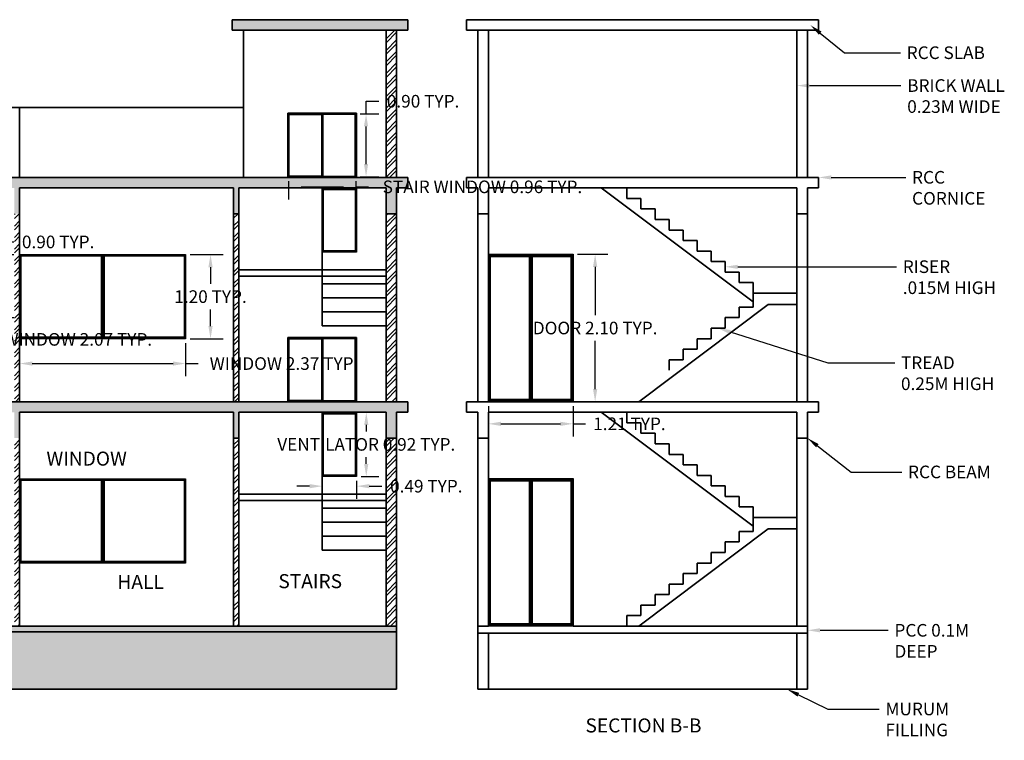
# Model space of a CAD drawing. Units: metres. Extents: x 8.1 to 56.2, y -9.3 to 36.3.
# Tile 5 of 6: x 22.5 to 36.6, y 25.7 to 36. Entities that reach past the tile are written whole.
import ezdxf
from ezdxf import colors
from ezdxf.entities.mleader import LeaderData, LeaderLine
from ezdxf.math import Vec2, Vec3

# ---------------------------------------------------------------- set-up
doc = ezdxf.new("R2010")
doc.units = ezdxf.units.M
doc.header["$LTSCALE"] = 0.01
doc.header["$MEASUREMENT"] = 0
for name, color, linetype, lineweight in [('A-ANNO-DIMS', 2, 'Continuous', 18), ('A-ANNO-TEXT', 7, 'Continuous', 18), ('A-DOOR', 4, 'Continuous', 25), ('A-GLAZ', 3, 'Continuous', 25), ('A-SECT', 7, 'Continuous', 35), ('A-SECT-PATT', 8, 'Continuous', 13)]:
    doc.layers.add(name, color=color, linetype=linetype, lineweight=lineweight)
doc.styles.get("Standard").update_dxf_attribs({"font": 'arial.ttf'})
doc.dimstyles.get("Standard").update_dxf_attribs({"dimtxt": 0.18, "dimasz": 0.18, "dimexe": 0.18, "dimexo": 0.0625, "dimgap": 0.09, "dimtad": 0, "dimtih": 1, "dimtoh": 1, "dimzin": 0, "dimdsep": 46, "dimtxsty": 'Standard', "dimcen": 0.09, "dimadec": 0, "dimazin": 0, "dimtfac": 1, "dimtofl": 0, "dimtmove": 0, "dimatfit": 3, "dimfxl": 1, "dimtolj": 1, "dimtzin": 0, "dimarcsym": 0})
pattern_1 = [(0, (-2.197816, 0), (0.023, 0.023), [0.0115, -0.0345]), (90, (-2.192066, -0.00575), (-0.023, 0.023), [0.0115, -0.0345])]
pattern_2 = [(0, (-2.197816, 0), (0.0235, 0.0235), [0.01175, -0.03525]), (90, (-2.19194, -0.005875), (-0.0235, 0.0235), [0.01175, -0.03525])]
pattern_3 = [(45, (-2.19782, 0), (-0.08220116, 0.08220116), []), (45, (-2.14301, 0), (-0.08220116, 0.08220116), [])]

# ---------------------------------------------------------------- blocks, each defined once
blk = doc.blocks.new('WIN-2400')
for p, q in [((1.164, 1.18), (1.164, 0.02)), ((1.174, 1.18), (1.174, 0.02)), ((1.184, 1.18), (1.184, 0.02)), ((1.194, 1.18), (1.194, 0.02)), ((1.204, 1.18), (1.204, 0.02))]:
    blk.add_line(p, q)
for points in [[(0, 1.2), (2.367, 1.2), (2.367, 0), (0, 0)], [(0.01, 1.19), (2.357, 1.19), (2.357, 0.01), (0.01, 0.01)], [(0.02, 1.18), (2.347, 1.18), (2.347, 0.02), (0.02, 0.02)]]:
    blk.add_lwpolyline(points, close=True)
blk = doc.blocks.new('WIN-VENT')
for points in [[(0, 0.916), (0.491, 0.916), (0.491, 0), (0, 0)], [(0.01, 0.906), (0.481, 0.906), (0.481, 0.01), (0.01, 0.01)], [(0.02, 0.896), (0.471, 0.896), (0.471, 0.02), (0.02, 0.02)]]:
    blk.add_lwpolyline(points, close=True)
blk = doc.blocks.new('DOOR-ELEV-1200')
for p, q in [((0.584, 2.074), (0.584, 0.03)), ((0.594, 2.074), (0.594, 0.03)), ((0.604, 2.074), (0.604, 0.03)), ((0.614, 2.074), (0.614, 0.03)), ((0.624, 2.074), (0.624, 0.03))]:
    blk.add_line(p, q)
for points in [[(1.208, 0), (0, 0), (0, 2.104), (1.208, 2.104)], [(1.198, 0.01), (0.01, 0.01), (0.01, 2.094), (1.198, 2.094)], [(1.188, 0.02), (0.02, 0.02), (0.02, 2.084), (1.188, 2.084)], [(1.178, 0.03), (0.03, 0.03), (0.03, 2.074), (1.178, 2.074)]]:
    blk.add_lwpolyline(points, close=True)
blk = doc.blocks.new('WIN-STAIR')
for p, q in [((0, 0), (0, 0.897)), ((0, 0.897), (0.47, 0.897)), ((0.01, 0.01), (0.01, 0.887)), ((0.01, 0.887), (0.46, 0.887)), ((0.47, 0.897), (0.47, 0.01)), ((0.961, 0.897), (0.49, 0.897)), ((0.49, 0.897), (0.49, 0.01)), ((0.951, 0.887), (0.5, 0.887)), ((0.951, 0.01), (0.951, 0.887)), ((0.961, 0), (0.961, 0.897)), ((0.47, 0), (0, 0)), ((0.46, 0.01), (0.01, 0.01)), ((0.46, 0.01), (0.951, 0.01)), ((0.47, 0), (0.961, 0))]:
    blk.add_line(p, q)
blk = doc.blocks.new('*D37')
at = {"layer": 'A-ANNO-DIMS', "color": 0, "lineweight": -2, "ltscale": 0.01, "transparency": 16777216}
for p, q in [((19.863, 31.647), (19.863, 31.219)), ((21.934, 31.647), (21.934, 31.219)), ((20.043, 31.399), (21.754, 31.399)), ((21.934, 31.399), (22.114, 31.399))]:
    blk.add_line(p, q, dxfattribs=at)
at = {"layer": 'A-ANNO-DIMS', "color": 0, "ltscale": 0.01, "transparency": 16777216}
for points in [[(20.043, 31.429), (20.043, 31.369), (19.863, 31.399)], [(21.754, 31.429), (21.754, 31.369), (21.934, 31.399)]]:
    blk.add_solid(points, dxfattribs=at)
at = {"layer": 'Defpoints', "color": 0, "ltscale": 0.01, "transparency": 16777216}
for p in [(19.863, 31.709), (21.934, 31.709), (21.934, 31.399)]:
    blk.add_point(p, dxfattribs=at)
at = {"layer": 'A-ANNO-DIMS', "color": 0, "ltscale": 0.01, "transparency": 16777216, "insert": (23.337, 31.399), "char_height": 0.18, "attachment_point": 5}
blk.add_mtext('\\A1;WINDOW 2.07 TYP.', dxfattribs=at)
blk = doc.blocks.new('*D38')
at = {"layer": 'A-ANNO-DIMS', "color": 0, "lineweight": -2, "ltscale": 0.01, "transparency": 16777216}
for p, q in [((22.244, 32.609), (22.244, 32.789)), ((22.244, 32.789), (22.424, 32.789)), ((21.996, 32.609), (22.424, 32.609)), ((22.244, 31.889), (22.244, 32.429)), ((21.996, 31.709), (22.424, 31.709))]:
    blk.add_line(p, q, dxfattribs=at)
at = {"layer": 'A-ANNO-DIMS', "color": 0, "ltscale": 0.01, "transparency": 16777216}
for points in [[(22.214, 32.429), (22.274, 32.429), (22.244, 32.609)], [(22.214, 31.889), (22.274, 31.889), (22.244, 31.709)]]:
    blk.add_solid(points, dxfattribs=at)
at = {"layer": 'Defpoints', "color": 0, "ltscale": 0.01, "transparency": 16777216}
for p in [(21.934, 32.609), (22.244, 32.609), (21.934, 31.709)]:
    blk.add_point(p, dxfattribs=at)
at = {"layer": 'A-ANNO-DIMS', "color": 0, "ltscale": 0.01, "transparency": 16777216, "insert": (23.057, 32.789), "char_height": 0.18, "attachment_point": 5}
blk.add_mtext('\\A1;0.90 TYP.', dxfattribs=at)
blk = doc.blocks.new('*D39')
at = {"layer": 'A-ANNO-DIMS', "color": 0, "lineweight": -2, "ltscale": 0.01, "transparency": 16777216}
for p, q in [((22.508, 31.347), (22.508, 30.874)), ((24.875, 31.347), (24.875, 30.874)), ((22.688, 31.054), (24.695, 31.054)), ((24.875, 31.054), (25.055, 31.054))]:
    blk.add_line(p, q, dxfattribs=at)
at = {"layer": 'A-ANNO-DIMS', "color": 0, "ltscale": 0.01, "transparency": 16777216}
for points in [[(22.688, 31.084), (22.688, 31.024), (22.508, 31.054)], [(24.695, 31.084), (24.695, 31.024), (24.875, 31.054)]]:
    blk.add_solid(points, dxfattribs=at)
at = {"layer": 'Defpoints', "color": 0, "ltscale": 0.01, "transparency": 16777216}
for p in [(22.508, 31.409), (24.875, 31.409), (24.875, 31.054)]:
    blk.add_point(p, dxfattribs=at)
at = {"layer": 'A-ANNO-DIMS', "color": 0, "ltscale": 0.01, "transparency": 16777216, "insert": (26.278, 31.054), "char_height": 0.18, "attachment_point": 5}
blk.add_mtext('\\A1;WINDOW 2.37 TYP.', dxfattribs=at)
blk = doc.blocks.new('*D40')
at = {"layer": 'A-ANNO-DIMS', "color": 0, "lineweight": -2, "ltscale": 0.01, "transparency": 16777216}
for p, q in [((24.938, 32.609), (25.41, 32.609)), ((25.23, 32.429), (25.23, 32.191)), ((25.23, 31.589), (25.23, 31.827)), ((24.938, 31.409), (25.41, 31.409))]:
    blk.add_line(p, q, dxfattribs=at)
at = {"layer": 'A-ANNO-DIMS', "color": 0, "ltscale": 0.01, "transparency": 16777216}
for points in [[(25.2, 32.429), (25.26, 32.429), (25.23, 32.609)], [(25.2, 31.589), (25.26, 31.589), (25.23, 31.409)]]:
    blk.add_solid(points, dxfattribs=at)
at = {"layer": 'Defpoints', "color": 0, "ltscale": 0.01, "transparency": 16777216}
for p in [(24.875, 32.609), (25.23, 32.609), (24.875, 31.409)]:
    blk.add_point(p, dxfattribs=at)
at = {"layer": 'A-ANNO-DIMS', "color": 0, "ltscale": 0.01, "transparency": 16777216, "insert": (25.23, 32.009), "char_height": 0.18, "attachment_point": 5}
blk.add_mtext('\\A1;1.20 TYP.', dxfattribs=at)
blk = doc.blocks.new('*D41')
at = {"layer": 'A-ANNO-DIMS', "color": 0, "lineweight": -2, "ltscale": 0.01, "transparency": 16777216}
for p, q in [((27.376, 30.359), (27.631, 30.359)), ((27.451, 30.179), (27.451, 30.084)), ((27.451, 29.623), (27.451, 29.718)), ((27.376, 29.443), (27.631, 29.443))]:
    blk.add_line(p, q, dxfattribs=at)
at = {"layer": 'A-ANNO-DIMS', "color": 0, "ltscale": 0.01, "transparency": 16777216}
for points in [[(27.421, 30.179), (27.481, 30.179), (27.451, 30.359)], [(27.421, 29.623), (27.481, 29.623), (27.451, 29.443)]]:
    blk.add_solid(points, dxfattribs=at)
at = {"layer": 'Defpoints', "color": 0, "ltscale": 0.01, "transparency": 16777216}
for p in [(27.314, 30.359), (27.451, 30.359), (27.314, 29.443)]:
    blk.add_point(p, dxfattribs=at)
at = {"layer": 'A-ANNO-DIMS', "color": 0, "ltscale": 0.01, "transparency": 16777216, "insert": (27.451, 29.901), "char_height": 0.18, "attachment_point": 5}
blk.add_mtext('\\A1;VENTILATOR 0.92 TYP.', dxfattribs=at)
blk = doc.blocks.new('*D42')
at = {"layer": 'A-ANNO-DIMS', "color": 0, "lineweight": -2, "ltscale": 0.01, "transparency": 16777216}
for p, q in [((26.823, 29.38), (26.823, 29.125)), ((27.314, 29.38), (27.314, 29.125)), ((26.643, 29.305), (26.463, 29.305)), ((27.494, 29.305), (27.674, 29.305))]:
    blk.add_line(p, q, dxfattribs=at)
at = {"layer": 'A-ANNO-DIMS', "color": 0, "ltscale": 0.01, "transparency": 16777216}
for points in [[(26.643, 29.335), (26.643, 29.275), (26.823, 29.305)], [(27.494, 29.335), (27.494, 29.275), (27.314, 29.305)]]:
    blk.add_solid(points, dxfattribs=at)
at = {"layer": 'Defpoints', "color": 0, "ltscale": 0.01, "transparency": 16777216}
for p in [(26.823, 29.443), (27.314, 29.443), (27.314, 29.305)]:
    blk.add_point(p, dxfattribs=at)
at = {"layer": 'A-ANNO-DIMS', "color": 0, "ltscale": 0.01, "transparency": 16777216, "insert": (28.307, 29.305), "char_height": 0.18, "attachment_point": 5}
blk.add_mtext('\\A1;0.49 TYP.', dxfattribs=at)
blk = doc.blocks.new('*D43')
at = {"layer": 'A-ANNO-DIMS', "color": 0, "lineweight": -2, "ltscale": 0.01, "transparency": 16777216}
for p, q in [((26.343, 33.657), (26.343, 33.395)), ((26.523, 33.575), (27.124, 33.575)), ((27.304, 33.657), (27.304, 33.395)), ((27.304, 33.575), (27.484, 33.575))]:
    blk.add_line(p, q, dxfattribs=at)
at = {"layer": 'A-ANNO-DIMS', "color": 0, "ltscale": 0.01, "transparency": 16777216}
for points in [[(26.523, 33.605), (26.523, 33.545), (26.343, 33.575)], [(27.124, 33.605), (27.124, 33.545), (27.304, 33.575)]]:
    blk.add_solid(points, dxfattribs=at)
at = {"layer": 'Defpoints', "color": 0, "ltscale": 0.01, "transparency": 16777216}
for p in [(26.343, 33.719), (27.304, 33.719), (27.304, 33.575)]:
    blk.add_point(p, dxfattribs=at)
at = {"layer": 'A-ANNO-DIMS', "color": 0, "ltscale": 0.01, "transparency": 16777216, "insert": (29.108, 33.575), "char_height": 0.18, "attachment_point": 5}
blk.add_mtext('\\A1;STAIR WINDOW 0.96 TYP.', dxfattribs=at)
blk = doc.blocks.new('*D44')
at = {"layer": 'A-ANNO-DIMS', "color": 0, "lineweight": -2, "ltscale": 0.01, "transparency": 16777216}
for p, q in [((27.448, 34.616), (27.448, 34.796)), ((27.448, 34.796), (27.628, 34.796)), ((27.366, 34.616), (27.628, 34.616)), ((27.448, 33.899), (27.448, 34.436)), ((27.366, 33.719), (27.628, 33.719))]:
    blk.add_line(p, q, dxfattribs=at)
at = {"layer": 'A-ANNO-DIMS', "color": 0, "ltscale": 0.01, "transparency": 16777216}
for points in [[(27.418, 34.436), (27.478, 34.436), (27.448, 34.616)], [(27.418, 33.899), (27.478, 33.899), (27.448, 33.719)]]:
    blk.add_solid(points, dxfattribs=at)
at = {"layer": 'Defpoints', "color": 0, "ltscale": 0.01, "transparency": 16777216}
for p in [(27.304, 34.616), (27.448, 34.616), (27.304, 33.719)]:
    blk.add_point(p, dxfattribs=at)
at = {"layer": 'A-ANNO-DIMS', "color": 0, "ltscale": 0.01, "transparency": 16777216, "insert": (28.261, 34.796), "char_height": 0.18, "attachment_point": 5}
blk.add_mtext('\\A1;0.90 TYP.', dxfattribs=at)
blk = doc.blocks.new('*D45')
at = {"layer": 'A-ANNO-DIMS', "color": 0, "lineweight": -2, "ltscale": 0.01, "transparency": 16777216}
for p, q in [((30.462, 32.613), (30.895, 32.613)), ((30.715, 32.433), (30.715, 31.744)), ((30.715, 30.689), (30.715, 31.378)), ((30.462, 30.509), (30.895, 30.509))]:
    blk.add_line(p, q, dxfattribs=at)
at = {"layer": 'A-ANNO-DIMS', "color": 0, "ltscale": 0.01, "transparency": 16777216}
for points in [[(30.685, 32.433), (30.745, 32.433), (30.715, 32.613)], [(30.685, 30.689), (30.745, 30.689), (30.715, 30.509)]]:
    blk.add_solid(points, dxfattribs=at)
at = {"layer": 'Defpoints', "color": 0, "ltscale": 0.01, "transparency": 16777216}
for p in [(30.4, 32.613), (30.715, 32.613), (30.4, 30.509)]:
    blk.add_point(p, dxfattribs=at)
at = {"layer": 'A-ANNO-DIMS', "color": 0, "ltscale": 0.01, "transparency": 16777216, "insert": (30.715, 31.561), "char_height": 0.18, "attachment_point": 5}
blk.add_mtext('\\A1;DOOR 2.10 TYP.', dxfattribs=at)
blk = doc.blocks.new('*D46')
at = {"layer": 'A-ANNO-DIMS', "color": 0, "lineweight": -2, "ltscale": 0.01, "transparency": 16777216}
for p, q in [((29.192, 30.447), (29.192, 30.014)), ((30.4, 30.447), (30.4, 30.014)), ((29.372, 30.194), (30.22, 30.194)), ((30.4, 30.194), (30.58, 30.194))]:
    blk.add_line(p, q, dxfattribs=at)
at = {"layer": 'A-ANNO-DIMS', "color": 0, "ltscale": 0.01, "transparency": 16777216}
for points in [[(29.372, 30.224), (29.372, 30.164), (29.192, 30.194)], [(30.22, 30.224), (30.22, 30.164), (30.4, 30.194)]]:
    blk.add_solid(points, dxfattribs=at)
at = {"layer": 'Defpoints', "color": 0, "ltscale": 0.01, "transparency": 16777216}
for p in [(29.192, 30.509), (30.4, 30.509), (30.4, 30.194)]:
    blk.add_point(p, dxfattribs=at)
at = {"layer": 'A-ANNO-DIMS', "color": 0, "ltscale": 0.01, "transparency": 16777216, "insert": (31.204, 30.194), "char_height": 0.18, "attachment_point": 5}
blk.add_mtext('\\A1;1.21 TYP.', dxfattribs=at)

msp = doc.modelspace()

# ---------------------------------------------------------------- hatches: boundary and pattern name
at = {"layer": 'A-SECT-PATT'}
h = msp.add_hatch(dxfattribs=at)
h.set_pattern_fill('CROSS', color=256, scale=0.094)
h.set_pattern_definition(pattern_2)
h.paths.add_polyline_path([(25.701, 35.959), (25.54, 35.959), (25.54, 35.809), (25.701, 35.809), (27.883, 35.809), (28.044, 35.809), (28.044, 35.959), (27.883, 35.959)])
h = msp.add_hatch(dxfattribs=at)
h.set_pattern_fill('ANSI32', color=256, scale=0.31)
h.set_pattern_definition(pattern_3)
h.paths.add_polyline_path([(27.733, 33.709), (27.883, 33.709), (27.883, 35.809), (27.733, 35.809)])
h = msp.add_hatch(dxfattribs=at)
h.set_pattern_fill('CROSS', color=256, scale=0.094)
h.set_pattern_definition(pattern_2)
h.paths.add_polyline_path([(15.663, 33.709), (15.503, 33.709), (15.503, 33.559), (15.663, 33.559), (15.663, 33.192), (15.813, 33.192), (15.813, 33.559), (17.013, 33.559), (17.013, 33.192), (17.088, 33.192), (17.088, 33.559), (19.788, 33.559), (19.788, 33.192), (19.863, 33.192), (19.863, 33.559), (22.433, 33.559), (22.433, 33.192), (22.508, 33.192), (22.508, 33.559), (25.558, 33.559), (25.558, 33.192), (25.633, 33.192), (25.633, 33.559), (27.733, 33.559), (27.733, 33.192), (27.883, 33.192), (27.883, 33.559), (28.044, 33.559), (28.044, 33.709), (27.883, 33.709)])
h = msp.add_hatch(dxfattribs=at)
h.set_pattern_fill('ANSI32', color=256, scale=0.31)
h.set_pattern_definition(pattern_3)
h.paths.add_polyline_path([(19.863, 33.192), (19.788, 33.192), (19.788, 30.509), (19.863, 30.509)])
h.paths.add_polyline_path([(22.508, 33.192), (22.433, 33.192), (22.433, 30.509), (22.508, 30.509)])
h.paths.add_polyline_path([(25.633, 33.192), (25.558, 33.192), (25.558, 30.509), (25.633, 30.509)])
h.paths.add_polyline_path([(27.883, 33.192), (27.733, 33.192), (27.733, 30.509), (27.883, 30.509)])
h.paths.add_polyline_path([(27.733, 27.309), (27.883, 27.309), (27.883, 29.992), (27.733, 29.992)])
h.paths.add_polyline_path([(25.558, 27.309), (25.633, 27.309), (25.633, 29.992), (25.558, 29.992)])
h = msp.add_hatch(dxfattribs=at)
h.set_pattern_fill('CROSS', color=256, scale=0.092)
h.set_pattern_definition(pattern_1)
h.paths.add_polyline_path([(17.013, 30.359), (17.013, 29.992), (17.088, 29.992), (17.088, 30.359), (19.788, 30.359), (19.788, 29.992), (19.863, 29.992), (19.863, 30.359), (22.433, 30.359), (22.433, 29.992), (22.508, 29.992), (22.508, 30.359), (25.558, 30.359), (25.558, 29.992), (25.633, 29.992), (25.633, 30.359), (27.733, 30.359), (27.733, 29.992), (27.883, 29.992), (27.883, 30.359), (28.044, 30.359), (28.044, 30.509), (27.883, 30.509), (15.663, 30.509), (15.503, 30.509), (15.503, 30.359), (15.663, 30.359), (15.663, 29.992), (15.813, 29.992), (15.813, 30.359)])
h = msp.add_hatch(dxfattribs=at)
h.set_pattern_fill('ANSI32', color=256, scale=0.31)
h.set_pattern_definition(pattern_3)
h.paths.add_polyline_path([(22.433, 27.309), (22.508, 27.309), (22.508, 29.992), (22.433, 29.992)])
h.paths.add_polyline_path([(19.788, 27.309), (19.863, 27.309), (19.863, 29.992), (19.788, 29.992)])
h.paths.add_polyline_path([(17.013, 27.309), (17.088, 27.309), (17.088, 29.992), (17.013, 29.992)])
h.paths.add_polyline_path([(15.663, 27.309), (15.813, 27.309), (15.813, 29.992), (15.663, 29.992)])
h = msp.add_hatch(dxfattribs=at)
h.set_pattern_fill('CROSS', color=256, scale=0.092)
h.set_pattern_definition(pattern_1)
h.paths.add_polyline_path([(15.663, 27.309), (15.663, 27.229), (27.883, 27.229), (27.883, 27.309)])
h = msp.add_hatch(dxfattribs=at)
h.set_pattern_fill('GRAVEL', color=256, scale=0.7)
h.set_pattern_definition([(228.01279, (-1.693816, 0.7), (-5.6, -6.3), [0.094175, -9.323362]), (184.96974, (-1.756816, 0.63), (8.4, 0.7), [0.161608, -15.999147]), (132.51045, (-1.917816, 0.616), (7, -7.7), [0.113952, -11.281223]), (267.27369, (-2.190816, 0.441), (0.7, 14), [0.147167, -14.569491]), (292.83365, (-2.197816, 0.294), (-3.5, 8.4), [0.1443085, -14.286561]), (357.27369, (-2.141816, 0.161), (-14, 0.7), [0.147167, -14.569491]), (37.69424, (-1.994816, 0.154), (-9.1, -7), [0.19462, -19.267394]), (72.25533, (-1.840816, 0.273), (4.9, 15.4), [0.183742, -18.190425]), (121.42957, (-1.784816, 0.448), (-5.6, 9.1), [0.147665, -14.618851]), (175.23636, (-1.861816, 0.574), (7.7, -0.7), [0.168582, -8.260534]), (222.39744, (-2.029816, 0.588), (-8.4, -7.7), [0.2180136, -21.5833625]), (138.81407, (-1.497816, 0.434), (-4.9, 4.2), [0.074411, -7.366691]), (171.46923, (-1.553816, 0.483), (9.1, -1.4), [0.141566, -14.015058]), (225, (-1.6938, 0.504), (-1e-16, -0.7), [0.098995, -0.890955]), (203.1986, (-1.74282, 0.588), (3.5, 1.4), [0.053311, -5.277731]), (291.8014, (-1.79182, 0.567), (-0.7, 2.1), [0.075392, -3.694223]), (30.96376, (-1.76382, 0.497), (2.1, 1.4), [0.12245, -3.959216]), (161.56505, (-1.65882, 0.56), (1.4, -0.7), [0.088544, -2.125051]), (16.38954, (-2.197816, 0.567), (7, 2.1), [0.12404, -12.279992]), (70.34618, (-2.078816, 0.602), (-2.8, -7.7), [0.104063, -10.302185]), (293.1986, (-1.65882, 0.7), (-1.4, 3.5), [0.10662, -5.224421]), (343.61046, (-1.616816, 0.602), (-7, 2.1), [0.12404, -12.279992]), (339.44395, (-2.197816, 0.133), (-3.5, 1.4), [0.119616, -5.861187]), (294.77514, (-2.085816, 0.091), (-3.5, 7.7), [0.100225, -9.92225]), (66.8014, (-1.65182, 0), (1.4, 3.5), [0.10662, -5.224421]), (17.35402, (-1.609816, 0.098), (-9.1, -2.8), [0.117342, -11.616797]), (69.44395, (-1.994816, 0), (-1.4, -3.5), [0.059808, -5.920995]), (101.30993, (-1.69382, 0), (-0.7, 2.8), [0.035693, -3.533621]), (165.96376, (-1.70082, 0.035), (2.1, -0.7), [0.144309, -2.741865]), (186.00901, (-1.840816, 0.07), (7, 0.7), [0.133735, -13.239746]), (303.69007, (-1.76382, 0.434), (-0.7, 1.4), [0.100955, -2.42293]), (353.15723, (-1.707816, 0.35), (11.9, -1.4), [0.176256, -17.449294]), (60.9454, (-1.532816, 0.329), (-2.8, -4.9), [0.072069, -7.134872]), (90, (-1.4978, 0.392), (-0.7, 0.7), [0.042, -0.658]), (120.25644, (-1.854816, 0.091), (2.8, -4.9), [0.097247, -9.627464]), (48.01279, (-1.903816, 0.175), (5.6, 6.3), [0.18835, -9.229186]), (0, (-1.7778, 0.315), (0.7, 0.7), [0.182, -0.518]), (325.30485, (-1.595816, 0.315), (7, -4.9), [0.11068, -10.957292]), (254.0546, (-1.50482, 0.252), (-0.7, -2.8), [0.101921, -4.994156]), (207.645975, (-1.532816, 0.154), (-13.3, -7), [0.1659455, -16.428632]), (175.42608, (-1.679816, 0.077), (-9.1, 0.7), [0.175559, -17.380351])])
h.paths.add_polyline_path([(27.883, 26.409), (27.883, 27.229), (15.663, 27.229), (15.663, 26.409)])

# ---------------------------------------------------------------- linework, layer by layer
at = {"layer": 'A-SECT'}
for p, q in [((25.701, 35.959), (25.54, 35.959)), ((25.54, 35.959), (25.54, 35.809)), ((27.883, 35.959), (25.701, 35.959)), ((27.883, 35.959), (28.044, 35.959)), ((28.044, 35.959), (28.044, 35.809)), ((29.042, 35.959), (28.881, 35.959)), ((28.881, 35.959), (28.881, 35.809)), ((33.742, 35.959), (29.042, 35.959)), ((33.742, 35.959), (33.902, 35.959)), ((33.902, 35.959), (33.902, 35.809)), ((25.54, 35.809), (25.701, 35.809)), ((25.701, 35.809), (25.701, 33.709)), ((27.883, 35.809), (25.701, 35.809)), ((27.733, 33.709), (27.733, 35.809)), ((27.883, 33.709), (27.883, 35.809)), ((28.044, 35.809), (27.883, 35.809)), ((28.881, 35.809), (29.042, 35.809)), ((29.042, 35.809), (29.042, 33.709)), ((33.742, 35.809), (29.042, 35.809)), ((29.192, 35.809), (29.192, 33.709)), ((33.592, 33.709), (33.592, 35.809)), ((33.742, 33.709), (33.742, 35.809)), ((33.902, 35.809), (33.742, 35.809)), ((15.663, 34.709), (25.701, 34.709)), ((22.508, 33.709), (22.508, 34.709)), ((26.333, 33.709), (26.333, 34.626)), ((26.333, 34.626), (26.823, 34.626)), ((27.314, 34.626), (26.823, 34.626)), ((26.823, 34.626), (26.823, 33.729)), ((26.823, 34.626), (26.823, 33.729)), ((27.314, 33.709), (27.314, 34.626)), ((15.663, 33.709), (27.883, 33.709)), ((27.883, 33.709), (28.044, 33.709)), ((28.044, 33.709), (28.044, 33.559)), ((29.042, 33.709), (28.881, 33.709)), ((28.881, 33.709), (28.881, 33.559)), ((29.042, 33.709), (33.742, 33.709)), ((33.742, 33.709), (33.902, 33.709)), ((33.902, 33.709), (33.902, 33.559)), ((22.508, 30.509), (22.508, 33.559)), ((22.508, 33.559), (25.558, 33.559)), ((25.558, 30.509), (25.558, 33.559)), ((25.633, 30.509), (25.633, 33.559)), ((25.633, 33.559), (27.733, 33.559)), ((26.823, 32.393), (26.823, 33.559)), ((27.733, 30.509), (27.733, 33.559)), ((27.883, 30.509), (27.883, 33.559)), ((28.044, 33.559), (27.883, 33.559)), ((28.881, 33.559), (29.042, 33.559)), ((29.042, 30.509), (29.042, 33.559)), ((29.192, 30.509), (29.192, 33.559)), ((29.192, 33.559), (33.592, 33.559)), ((31.169, 33.559), (31.169, 33.409)), ((33.592, 30.509), (33.592, 33.559)), ((33.742, 30.509), (33.742, 33.559)), ((33.902, 33.559), (33.742, 33.559)), ((31.169, 33.409), (31.369, 33.409)), ((31.369, 33.409), (31.369, 33.259)), ((25.558, 33.192), (25.633, 33.192)), ((27.733, 33.192), (27.883, 33.192)), ((29.042, 33.192), (29.192, 33.192)), ((31.369, 33.259), (31.569, 33.259)), ((31.569, 33.259), (31.569, 33.109)), ((33.592, 33.192), (33.742, 33.192)), ((31.569, 33.109), (31.769, 33.109)), ((31.769, 33.109), (31.769, 32.959)), ((31.769, 32.959), (31.969, 32.959)), ((31.969, 32.959), (31.969, 32.809)), ((31.969, 32.809), (32.169, 32.809)), ((32.169, 32.809), (32.169, 32.659)), ((32.169, 32.659), (32.369, 32.659)), ((32.369, 32.659), (32.369, 32.509)), ((32.369, 32.509), (32.569, 32.509)), ((32.569, 32.509), (32.569, 32.359)), ((26.823, 32.393), (25.633, 32.393)), ((27.733, 32.3), (25.633, 32.3)), ((27.733, 32.393), (26.823, 32.393)), ((26.823, 31.593), (26.823, 32.393)), ((32.569, 32.359), (32.769, 32.359)), ((32.769, 32.359), (32.769, 32.209)), ((27.733, 32.193), (26.823, 32.193)), ((32.769, 32.209), (32.969, 32.209)), ((32.969, 32.209), (32.969, 32.059)), ((32.969, 32.059), (33.592, 32.059)), ((32.969, 32.059), (32.969, 32.009)), ((27.733, 31.993), (26.823, 31.993)), ((32.969, 32.009), (32.969, 31.859)), ((33.184, 31.896), (33.592, 31.896)), ((27.733, 31.793), (26.823, 31.793)), ((32.969, 31.859), (32.769, 31.859)), ((32.769, 31.859), (32.769, 31.709)), ((32.769, 31.709), (32.569, 31.709)), ((32.569, 31.709), (32.569, 31.559)), ((27.733, 31.593), (26.823, 31.593)), ((32.569, 31.559), (32.369, 31.559)), ((32.369, 31.559), (32.369, 31.409)), ((26.333, 30.509), (26.333, 31.426)), ((26.333, 31.426), (26.823, 31.426)), ((27.314, 31.426), (26.823, 31.426)), ((26.823, 31.426), (26.823, 30.529)), ((26.823, 31.426), (26.823, 30.529)), ((27.314, 30.509), (27.314, 31.426)), ((32.369, 31.409), (32.169, 31.409)), ((32.169, 31.409), (32.169, 31.259)), ((32.169, 31.259), (31.969, 31.259)), ((31.969, 31.259), (31.969, 31.109)), ((31.969, 31.109), (31.769, 31.109)), ((31.769, 31.109), (31.769, 30.959)), ((15.663, 30.509), (27.883, 30.509)), ((26.823, 30.509), (26.333, 30.509)), ((26.823, 30.509), (27.314, 30.509)), ((27.883, 30.509), (28.044, 30.509)), ((28.044, 30.509), (28.044, 30.359)), ((29.042, 30.509), (28.881, 30.509)), ((28.881, 30.509), (28.881, 30.359)), ((29.042, 30.509), (33.742, 30.509)), ((33.742, 30.509), (33.902, 30.509)), ((33.902, 30.509), (33.902, 30.359)), ((22.508, 27.309), (22.508, 30.359)), ((22.508, 30.359), (25.558, 30.359)), ((25.558, 27.309), (25.558, 30.359)), ((25.633, 27.309), (25.633, 30.359)), ((25.633, 30.359), (27.733, 30.359)), ((26.823, 29.193), (26.823, 30.359)), ((27.733, 27.309), (27.733, 30.359)), ((27.883, 27.309), (27.883, 30.359)), ((28.044, 30.359), (27.883, 30.359)), ((28.881, 30.359), (29.042, 30.359)), ((29.042, 27.309), (29.042, 30.359)), ((29.192, 27.309), (29.192, 30.359)), ((29.192, 30.359), (33.592, 30.359)), ((31.169, 30.359), (31.169, 30.209)), ((33.592, 27.309), (33.592, 30.359)), ((33.742, 27.309), (33.742, 30.359)), ((33.902, 30.359), (33.742, 30.359)), ((31.169, 30.209), (31.369, 30.209)), ((31.369, 30.209), (31.369, 30.059)), ((31.369, 30.059), (31.569, 30.059)), ((31.569, 30.059), (31.569, 29.909)), ((25.558, 29.992), (25.633, 29.992)), ((27.733, 29.992), (27.883, 29.992)), ((29.042, 29.992), (29.192, 29.992)), ((33.592, 29.992), (33.742, 29.992)), ((31.569, 29.909), (31.769, 29.909)), ((31.769, 29.909), (31.769, 29.759)), ((31.769, 29.759), (31.969, 29.759)), ((31.969, 29.759), (31.969, 29.609)), ((31.969, 29.609), (32.169, 29.609)), ((32.169, 29.609), (32.169, 29.459)), ((32.169, 29.459), (32.369, 29.459)), ((32.369, 29.459), (32.369, 29.309)), ((32.369, 29.309), (32.569, 29.309)), ((32.569, 29.309), (32.569, 29.159)), ((26.823, 29.193), (25.633, 29.193)), ((27.733, 29.1), (25.633, 29.1)), ((27.733, 29.193), (26.823, 29.193)), ((26.823, 28.393), (26.823, 29.193)), ((32.569, 29.159), (32.769, 29.159)), ((32.769, 29.159), (32.769, 29.009)), ((27.733, 28.993), (26.823, 28.993)), ((32.769, 29.009), (32.969, 29.009)), ((32.969, 29.009), (32.969, 28.859)), ((27.733, 28.793), (26.823, 28.793)), ((32.969, 28.859), (33.592, 28.859)), ((32.969, 28.859), (32.969, 28.809)), ((32.969, 28.809), (32.969, 28.659)), ((32.969, 28.659), (32.769, 28.659)), ((32.769, 28.659), (32.769, 28.509)), ((33.184, 28.696), (33.592, 28.696)), ((27.733, 28.593), (26.823, 28.593)), ((32.769, 28.509), (32.569, 28.509)), ((32.569, 28.509), (32.569, 28.359)), ((27.733, 28.393), (26.823, 28.393)), ((32.569, 28.359), (32.369, 28.359)), ((32.369, 28.359), (32.369, 28.209)), ((32.369, 28.209), (32.169, 28.209)), ((32.169, 28.209), (32.169, 28.059)), ((32.169, 28.059), (31.969, 28.059)), ((31.969, 28.059), (31.969, 27.909)), ((31.969, 27.909), (31.769, 27.909)), ((31.769, 27.909), (31.769, 27.759)), ((31.769, 27.759), (31.569, 27.759)), ((31.569, 27.759), (31.569, 27.609)), ((31.569, 27.609), (31.369, 27.609)), ((31.369, 27.609), (31.369, 27.459)), ((31.369, 27.459), (31.169, 27.459)), ((31.169, 27.459), (31.169, 27.309)), ((15.663, 27.309), (27.883, 27.309)), ((27.883, 27.309), (27.883, 26.409)), ((29.042, 26.409), (29.042, 27.309)), ((29.192, 27.309), (29.042, 27.309)), ((30.4, 27.309), (33.742, 27.309)), ((33.742, 27.309), (33.742, 26.409)), ((15.663, 27.229), (27.883, 27.229)), ((29.042, 27.209), (33.742, 27.209)), ((29.192, 26.409), (29.192, 27.209)), ((33.592, 27.209), (33.592, 26.409)), ((15.663, 26.409), (27.883, 26.409)), ((29.042, 26.409), (33.742, 26.409))]:
    msp.add_line(p, q, dxfattribs=at)
for points in [[(30.802, 33.559), (32.969, 31.934)], [(33.184, 31.896), (31.336, 30.509)], [(30.802, 30.359), (32.969, 28.734)], [(33.184, 28.696), (31.336, 27.309)]]:
    msp.add_lwpolyline(points, dxfattribs=at)

# ---------------------------------------------------------------- block references
at = {"layer": 'A-DOOR'}
for p in [(29.192, 30.509), (29.192, 27.309)]:
    msp.add_blockref('DOOR-ELEV-1200', p, dxfattribs=at)
at = {"layer": 'A-GLAZ'}
for name, p in [('WIN-STAIR', (26.343, 33.719)), ('WIN-VENT', (26.823, 32.643)), ('WIN-2400', (22.508, 31.409)), ('WIN-STAIR', (26.343, 30.519)), ('WIN-VENT', (26.823, 29.443)), ('WIN-2400', (22.508, 28.209))]:
    msp.add_blockref(name, p, dxfattribs=at)

# ---------------------------------------------------------------- texts
at = {"layer": 'A-ANNO-TEXT', "char_height": 0.2, "attachment_point": 1}
for s, width, insert in [('WINDOW', 1.61769, (22.89, 29.798)), ('\\pxqc;HALL', 1.61769, (23.424, 28.04)), ('\\pxqc;STAIRS', 1.61769, (25.843, 28.05)), ('\\pxqc;SECTION B-B', 4.05553, (29.377, 25.992))]:
    msp.add_mtext_dynamic_manual_height_columns(s, width=width, gutter_width=1, heights=[0], dxfattribs=dict(at, insert=insert))

# ---------------------------------------------------------------- dimensions: what is measured, and where the dimension line sits
at = {"layer": 'A-ANNO-DIMS', "ltscale": 0.01}
for base, p1, p2, text, picture, middle in [((27.448, 34.616), (27.304, 33.719), (27.304, 34.616), '<> TYP.', '*D44', (28.261, 34.796)), ((22.244, 32.609), (21.934, 31.709), (21.934, 32.609), '<> TYP.', '*D38', (23.057, 32.789)), ((25.23, 32.609), (24.875, 31.409), (24.875, 32.609), '<> TYP.', '*D40', (25.23, 32.009)), ((30.715, 32.613), (30.4, 30.509), (30.4, 32.613), 'DOOR <> TYP.', '*D45', (30.715, 31.561)), ((27.451, 30.359), (27.314, 29.443), (27.314, 30.359), 'VENTILATOR <> TYP.', '*D41', (27.451, 29.901))]:
    dim = msp.add_linear_dim(base=base, p1=p1, p2=p2, angle=90, text=text, dimstyle='Standard', override={"dimdec": 2, "dimrnd": 0, "dimzin": 0, "dimlunit": 2}, dxfattribs=at)
    dim.commit()
    dim.dimension.update_dxf_attribs({"geometry": picture, "text_midpoint": middle})
for base, p1, p2, text, picture, middle in [((27.304, 33.575), (26.343, 33.719), (27.304, 33.719), 'STAIR WINDOW <> TYP.', '*D43', (29.108, 33.575)), ((21.934, 31.399), (19.863, 31.709), (21.934, 31.709), 'WINDOW <> TYP.', '*D37', (23.337, 31.399)), ((24.875, 31.054), (22.508, 31.409), (24.875, 31.409), 'WINDOW <> TYP.', '*D39', (26.278, 31.054)), ((30.4, 30.194), (29.192, 30.509), (30.4, 30.509), '<> TYP.', '*D46', (31.204, 30.194)), ((27.314, 29.305), (26.823, 29.443), (27.314, 29.443), '<> TYP.', '*D42', (28.307, 29.305))]:
    dim = msp.add_linear_dim(base=base, p1=p1, p2=p2, text=text, dimstyle='Standard', override={"dimdec": 2, "dimrnd": 0, "dimzin": 0, "dimlunit": 2}, dxfattribs=at)
    dim.commit()
    dim.dimension.update_dxf_attribs({"geometry": picture, "text_midpoint": middle})

# ---------------------------------------------------------------- leaders
at = {"layer": 'A-ANNO-TEXT'}
ml = msp.add_multileader_mtext('Standard', dxfattribs=at)
ml.set_content('RCC SLAB', color=256)
ml.set_leader_properties()
ml.build(insert=Vec2(0, 0))
ml.multileader.update_dxf_attribs({"dogleg_length": 0.36, "arrow_head_size": 0.18})
ctx = ml.context
ctx.base_point, ctx.char_height, ctx.arrow_head_size, ctx.landing_gap_size, ctx.plane_origin = Vec3(35.069, 35.487), 0.18, 0.18, 0.09, Vec3(33.785, 35.881)
notes = []
notes.append((ctx, [(0, (1, 1, 0), (34.709, 35.487), (1, 0), 0.36, [(0, [(33.785, 35.881), (34.271, 35.487)], 0, [])])]))
ctx.mtext.insert, ctx.mtext.flow_direction = Vec3(35.159, 35.578), 5
ml = msp.add_multileader_mtext('Standard', dxfattribs=at)
ml.set_content('BRICK WALL\\P0.23M WIDE', color=256)
ml.set_leader_properties()
ml.build(insert=Vec2(0, 0))
ml.multileader.update_dxf_attribs({"dogleg_length": 0.36, "arrow_head_size": 0.18})
ctx = ml.context
ctx.base_point, ctx.char_height, ctx.arrow_head_size, ctx.landing_gap_size, ctx.plane_origin = Vec3(35.076, 35.019), 0.18, 0.18, 0.09, Vec3(33.592, 35.019)
notes.append((ctx, [(0, (1, 1, 0), (34.716, 35.019), (1, 0), 0.36, [(0, [(33.592, 35.019), (34.271, 35.019)], 0, [])])]))
ctx.mtext.insert, ctx.mtext.flow_direction = Vec3(35.166, 35.11), 5
ml = msp.add_multileader_mtext('Standard', dxfattribs=at)
ml.set_content('RCC\\PCORNICE', color=256)
ml.set_leader_properties()
ml.build(insert=Vec2(0, 0))
ml.multileader.update_dxf_attribs({"dogleg_length": 0.36, "arrow_head_size": 0.18})
ctx = ml.context
ctx.base_point, ctx.char_height, ctx.arrow_head_size, ctx.landing_gap_size, ctx.plane_origin = Vec3(35.145, 33.709), 0.18, 0.18, 0.09, Vec3(33.902, 33.709)
notes.append((ctx, [(0, (1, 1, 0), (34.785, 33.709), (1, 0), 0.36, [(0, [(33.902, 33.709), (34.704, 33.709)], 0, [])])]))
ctx.mtext.insert, ctx.mtext.flow_direction = Vec3(35.235, 33.801), 5
ml = msp.add_multileader_mtext('Standard', dxfattribs=at)
ml.set_content('RISER\\P.015M HIGH', color=256)
ml.set_leader_properties()
ml.build(insert=Vec2(0, 0))
ml.multileader.update_dxf_attribs({"dogleg_length": 0.36, "arrow_head_size": 0.18})
ctx = ml.context
ctx.base_point, ctx.char_height, ctx.arrow_head_size, ctx.landing_gap_size, ctx.plane_origin = Vec3(35.013, 32.434), 0.18, 0.18, 0.09, Vec3(32.569, 32.434)
notes.append((ctx, [(0, (1, 1, 0), (34.653, 32.434), (1, 0), 0.36, [(0, [(32.569, 32.434), (34.018, 32.434)], 0, [])])]))
ctx.mtext.insert, ctx.mtext.flow_direction = Vec3(35.103, 32.526), 5
ml = msp.add_multileader_mtext('Standard', dxfattribs=at)
ml.set_content('TREAD\\P0.25M HIGH', color=256)
ml.set_leader_properties()
ml.build(insert=Vec2(0, 0))
ml.multileader.update_dxf_attribs({"dogleg_length": 0.36, "arrow_head_size": 0.18})
ctx = ml.context
ctx.base_point, ctx.char_height, ctx.arrow_head_size, ctx.landing_gap_size, ctx.plane_origin = Vec3(34.987, 31.064), 0.18, 0.18, 0.09, Vec3(32.469, 31.559)
notes.append((ctx, [(0, (1, 1, 0), (34.627, 31.064), (1, 0), 0.36, [(0, [(32.469, 31.559), (34.033, 31.064)], 0, [])])]))
ctx.mtext.insert, ctx.mtext.flow_direction = Vec3(35.077, 31.156), 5
ml = msp.add_multileader_mtext('Standard', dxfattribs=at)
ml.set_content('RCC BEAM', color=256)
ml.set_leader_properties()
ml.build(insert=Vec2(0, 0))
ml.multileader.update_dxf_attribs({"dogleg_length": 0.36, "arrow_head_size": 0.18})
ctx = ml.context
ctx.base_point, ctx.char_height, ctx.arrow_head_size, ctx.landing_gap_size, ctx.plane_origin = Vec3(35.088, 29.507), 0.18, 0.18, 0.09, Vec3(33.742, 29.992)
notes.append((ctx, [(0, (1, 1, 0), (34.728, 29.507), (1, 0), 0.36, [(0, [(33.742, 29.992), (34.368, 29.507)], 0, [])])]))
ctx.mtext.insert, ctx.mtext.flow_direction = Vec3(35.178, 29.598), 5
ml = msp.add_multileader_mtext('Standard', dxfattribs=at)
ml.set_content('PCC 0.1M\\PDEEP', color=256)
ml.set_leader_properties()
ml.build(insert=Vec2(0, 0))
ml.multileader.update_dxf_attribs({"dogleg_length": 0.36, "arrow_head_size": 0.18})
ctx = ml.context
ctx.base_point, ctx.char_height, ctx.arrow_head_size, ctx.landing_gap_size, ctx.plane_origin = Vec3(34.894, 27.249), 0.18, 0.18, 0.09, Vec3(33.742, 27.249)
notes.append((ctx, [(0, (1, 1, 0), (34.534, 27.249), (1, 0), 0.36, [(0, [(33.742, 27.249), (34.322, 27.249)], 0, [])])]))
ctx.mtext.insert, ctx.mtext.flow_direction = Vec3(34.984, 27.339), 5
ml = msp.add_multileader_mtext('Standard', dxfattribs=at)
ml.set_content('MURUM\\PFILLING', color=256)
ml.set_leader_properties()
ml.build(insert=Vec2(0, 0))
ml.multileader.update_dxf_attribs({"dogleg_length": 0.36, "arrow_head_size": 0.18})
ctx = ml.context
ctx.base_point, ctx.char_height, ctx.arrow_head_size, ctx.landing_gap_size, ctx.plane_origin = Vec3(34.766, 26.125), 0.18, 0.18, 0.09, Vec3(33.452, 26.409)
notes.append((ctx, [(0, (1, 1, 0), (34.406, 26.125), (1, 0), 0.36, [(0, [(33.452, 26.409), (34.032, 26.125)], 0, [])])]))
ctx.mtext.insert, ctx.mtext.flow_direction = Vec3(34.856, 26.217), 5
for ctx, leaders in notes:
    for number, flags, end, landing, length, lines in leaders:
        leader = LeaderData()
        leader.index, (leader.has_last_leader_line, leader.has_dogleg_vector, leader.attachment_direction) = number, flags
        leader.last_leader_point, leader.dogleg_vector, leader.dogleg_length = Vec3(end), Vec3(landing), length
        for number, points, colour, breaks in lines:
            line = LeaderLine()
            line.index, line.vertices, line.color, line.breaks = number, Vec3.list(points), colors.encode_raw_color(colour), breaks
            leader.lines.append(line)
        ctx.leaders.append(leader)

doc.saveas('drawing.dxf')
